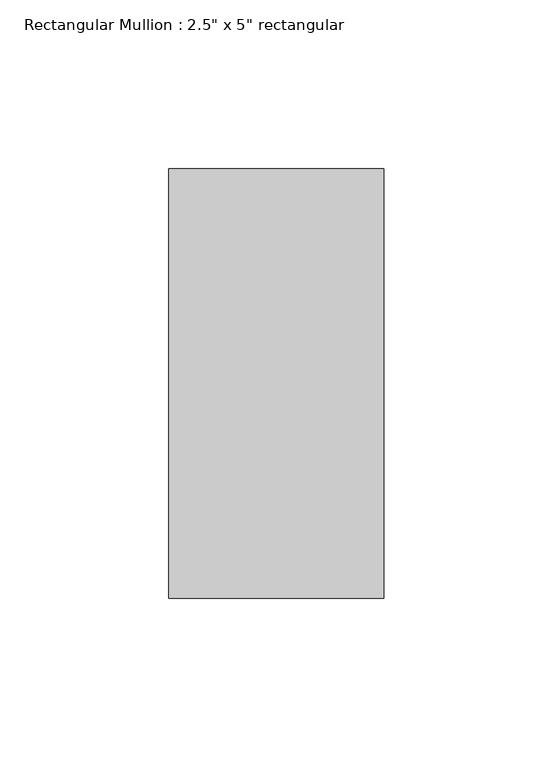
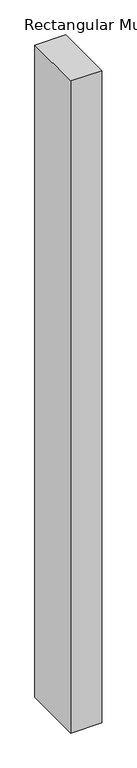
"""IFC4 building model written with IfcOpenShell, lengths in millimetres: member geometry."""

from ifc_helpers import new_model, si_unit, frame, origin, place, context, project, spatial, polyline, outline, extrude, source, transform, mapped, element, save


def member_243ec899(model_context):
    return source(origin(), model_context, "Body", "SweptSolid", [
        extrude(outline(polyline([(0.0, 63.5), (0.0, -63.5), (-63.5, -63.5), (-63.5, 63.5), (0.0, 63.5)])), frame((0.0, 0.0, -1409.7), z_axis=(0.0, 0.0, 1.0), x_axis=(1.0, 0.0, 0.0)), (0.0, 0.0, 1.0), 1409.7),
    ])


if __name__ == "__main__":
    model = new_model("IFC4")
    model_context = context("Model", 3, world=origin())
    ifc_project = project(units=[si_unit("LENGTHUNIT", "METRE", prefix="MILLI")], contexts=[model_context])
    site = spatial("IfcSite", under=ifc_project)
    building = spatial("IfcBuilding", under=site)
    placement = place(None, origin())
    member_shape = member_243ec899(model_context)
    element("IfcMember", 1, ObjectType="Rectangular Mullion : 2.5\" x 5\" rectangular", at=placement, inside=building, context=model_context, shape_type="MappedRepresentation", body=[
        mapped(member_shape, transform((0.0, 0.0, 0.0), x_axis=(1.0, 0.0, 0.0), y_axis=(0.0, 1.0, 0.0), z_axis=(0.0, 0.0, 1.0))),
    ])
    save(model, "model.ifc")

# Revit data of these elements
# Type "Rectangular Mullion : 2.5\" x 5\" rectangular"
#   built-in parameter 1007304 = 0.416667 (stored number, unit not read)
#   built-in parameter 1007301 = 0.104167 (stored number, unit not read)
#   built-in parameter 1007300 = 0.104167 (stored number, unit not read)
# Element 1 (IfcMember, "Rectangular Mullion : 2.5\" x 5\" rectangular")
#   Materials on its faces: "Aluminum"
# Materials
#   "Aluminum": class "Metal", colour RGB 247 247 247, transparency 0, Description = "Aluminum 6061", Cost = 0
